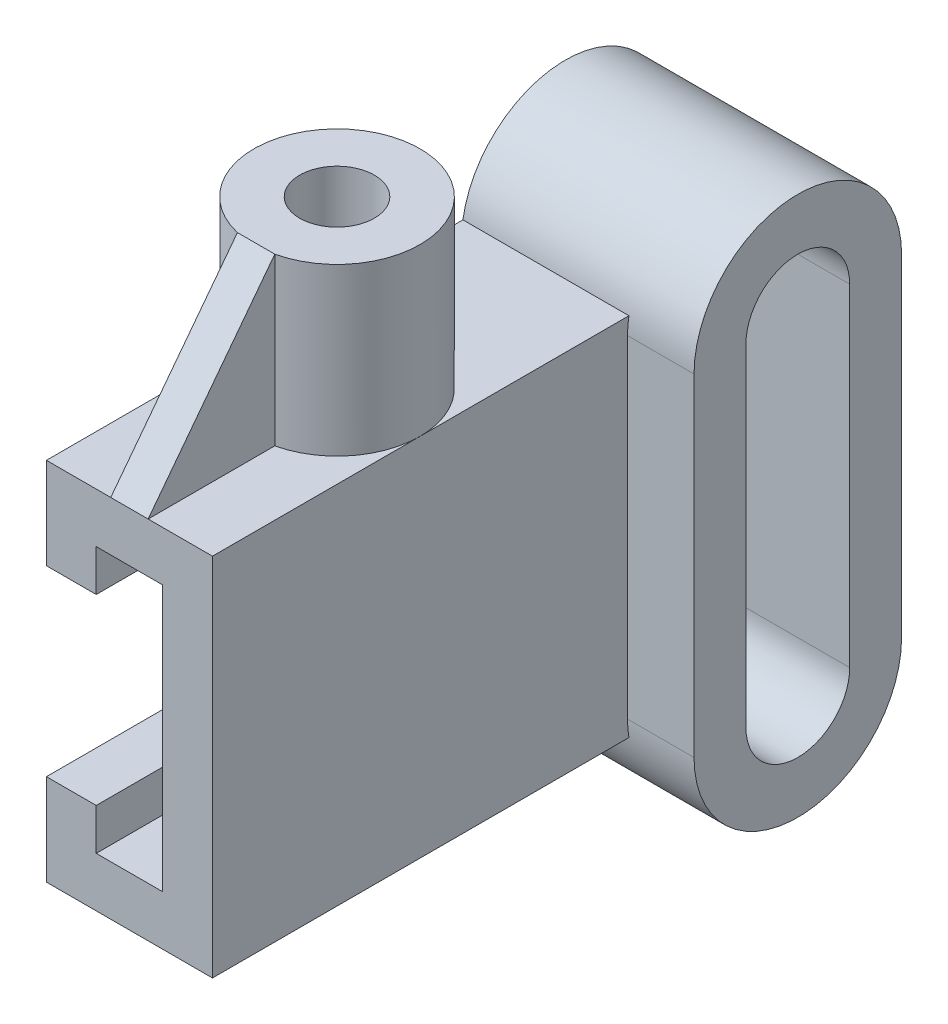
ISO-10303-21;
HEADER;
FILE_DESCRIPTION(('STEP AP214'),'2;1');
FILE_NAME('part.step','',(''),(''),'','','');
FILE_SCHEMA(('AUTOMOTIVE_DESIGN { 1 0 10303 214 1 1 1 1 }'));
ENDSEC;
DATA;
#1=APPLICATION_CONTEXT('core data for automotive mechanical design processes');
#2=APPLICATION_PROTOCOL_DEFINITION('international standard','automotive_design',2000,#1);
#3=PRODUCT_CONTEXT('',#1,'mechanical');
#4=PRODUCT('Part','Part','',(#3));
#5=PRODUCT_RELATED_PRODUCT_CATEGORY('part','',(#4));
#6=PRODUCT_DEFINITION_FORMATION('','',#4);
#7=PRODUCT_DEFINITION_CONTEXT('part definition',#1,'design');
#8=PRODUCT_DEFINITION('design','',#6,#7);
#9=PRODUCT_DEFINITION_SHAPE('','',#8);
#10=(LENGTH_UNIT() NAMED_UNIT(*) SI_UNIT(.MILLI.,.METRE.));
#11=(NAMED_UNIT(*) PLANE_ANGLE_UNIT() SI_UNIT($,.RADIAN.));
#12=(NAMED_UNIT(*) SI_UNIT($,.STERADIAN.) SOLID_ANGLE_UNIT());
#13=UNCERTAINTY_MEASURE_WITH_UNIT(LENGTH_MEASURE(1.E-05),#10,'distance_accuracy_value','');
#14=(GEOMETRIC_REPRESENTATION_CONTEXT(3) GLOBAL_UNCERTAINTY_ASSIGNED_CONTEXT((#13)) GLOBAL_UNIT_ASSIGNED_CONTEXT((#10,
#11,#12)) REPRESENTATION_CONTEXT('',''));
#15=CARTESIAN_POINT('',(0.,0.,0.));
#16=DIRECTION('',(0.,0.,1.));
#17=DIRECTION('',(1.,0.,0.));
#18=AXIS2_PLACEMENT_3D('',#15,#16,#17);
#19=CARTESIAN_POINT('',(-20.,-40.,-74.9999999999999));
#20=DIRECTION('',(1.,0.,0.));
#21=DIRECTION('',(0.,0.,-1.));
#22=AXIS2_PLACEMENT_3D('',#19,#20,#21);
#23=CYLINDRICAL_SURFACE('',#22,25.);
#24=CARTESIAN_POINT('',(20.,-40.,-74.9999999999999));
#25=DIRECTION('',(-1.,0.,0.));
#26=DIRECTION('',(0.,0.,1.));
#27=AXIS2_PLACEMENT_3D('',#24,#25,#26);
#28=CIRCLE('',#27,25.);
#29=CARTESIAN_POINT('',(20.,-44.,-50.3220746414938));
#30=VERTEX_POINT('',#29);
#31=CARTESIAN_POINT('',(20.,-40.,-50.));
#32=VERTEX_POINT('',#31);
#33=EDGE_CURVE('E11',#30,#32,#28,.T.);
#34=ORIENTED_EDGE('',*,*,#33,.F.);
#35=DIRECTION('',(1.,0.,0.));
#36=VECTOR('',#35,1.);
#37=CARTESIAN_POINT('',(-20.,-44.,-50.3220746414938));
#38=LINE('',#37,#36);
#39=CARTESIAN_POINT('',(-20.,-44.,-50.3220746414938));
#40=VERTEX_POINT('',#39);
#41=EDGE_CURVE('E47',#40,#30,#38,.T.);
#42=ORIENTED_EDGE('',*,*,#41,.F.);
#43=CARTESIAN_POINT('',(-20.,-40.,-74.9999999999999));
#44=DIRECTION('',(1.,0.,0.));
#45=DIRECTION('',(0.,0.,-1.));
#46=AXIS2_PLACEMENT_3D('',#43,#44,#45);
#47=CIRCLE('',#46,25.);
#48=CARTESIAN_POINT('',(-20.,-40.,-99.9999999999999));
#49=VERTEX_POINT('',#48);
#50=EDGE_CURVE('E340',#49,#40,#47,.F.);
#51=ORIENTED_EDGE('',*,*,#50,.F.);
#52=DIRECTION('',(1.,0.,0.));
#53=VECTOR('',#52,1.);
#54=CARTESIAN_POINT('',(-20.,-40.,-99.9999999999999));
#55=LINE('',#54,#53);
#56=CARTESIAN_POINT('',(36.,-40.,-99.9999999999999));
#57=VERTEX_POINT('',#56);
#58=EDGE_CURVE('E310',#49,#57,#55,.T.);
#59=ORIENTED_EDGE('',*,*,#58,.T.);
#60=CARTESIAN_POINT('',(36.,-40.,-74.9999999999999));
#61=DIRECTION('',(1.,0.,0.));
#62=DIRECTION('',(0.,0.,-1.));
#63=AXIS2_PLACEMENT_3D('',#60,#61,#62);
#64=CIRCLE('',#63,25.);
#65=CARTESIAN_POINT('',(36.,-40.,-50.));
#66=VERTEX_POINT('',#65);
#67=EDGE_CURVE('E349',#66,#57,#64,.T.);
#68=ORIENTED_EDGE('',*,*,#67,.F.);
#69=DIRECTION('',(-1.,0.,0.));
#70=VECTOR('',#69,1.);
#71=CARTESIAN_POINT('',(36.,-40.,-50.));
#72=LINE('',#71,#70);
#73=EDGE_CURVE('E219',#66,#32,#72,.T.);
#74=ORIENTED_EDGE('',*,*,#73,.T.);
#75=EDGE_LOOP('',(#34,#42,#51,#59,#68,#74));
#76=FACE_BOUND('',#75,.T.);
#77=ADVANCED_FACE('F41',(#76),#23,.T.);
#78=CARTESIAN_POINT('',(-20.,40.,-75.));
#79=DIRECTION('',(1.,0.,0.));
#80=DIRECTION('',(0.,0.,-1.));
#81=AXIS2_PLACEMENT_3D('',#78,#79,#80);
#82=CYLINDRICAL_SURFACE('',#81,25.);
#83=DIRECTION('',(1.,0.,0.));
#84=VECTOR('',#83,1.);
#85=CARTESIAN_POINT('',(-20.,44.,-50.3220746414938));
#86=LINE('',#85,#84);
#87=CARTESIAN_POINT('',(-20.,44.,-50.3220746414938));
#88=VERTEX_POINT('',#87);
#89=CARTESIAN_POINT('',(20.,44.,-50.3220746414938));
#90=VERTEX_POINT('',#89);
#91=EDGE_CURVE('E225',#88,#90,#86,.T.);
#92=ORIENTED_EDGE('',*,*,#91,.T.);
#93=CARTESIAN_POINT('',(20.,40.,-75.));
#94=DIRECTION('',(-1.,0.,0.));
#95=DIRECTION('',(0.,0.,1.));
#96=AXIS2_PLACEMENT_3D('',#93,#94,#95);
#97=CIRCLE('',#96,25.);
#98=CARTESIAN_POINT('',(20.,40.,-50.));
#99=VERTEX_POINT('',#98);
#100=EDGE_CURVE('E224',#90,#99,#97,.F.);
#101=ORIENTED_EDGE('',*,*,#100,.T.);
#102=DIRECTION('',(-1.,0.,0.));
#103=VECTOR('',#102,1.);
#104=CARTESIAN_POINT('',(36.,40.,-50.));
#105=LINE('',#104,#103);
#106=CARTESIAN_POINT('',(36.,40.,-50.));
#107=VERTEX_POINT('',#106);
#108=EDGE_CURVE('E339',#107,#99,#105,.T.);
#109=ORIENTED_EDGE('',*,*,#108,.F.);
#110=CARTESIAN_POINT('',(36.,40.,-75.));
#111=DIRECTION('',(1.,0.,0.));
#112=DIRECTION('',(0.,0.,-1.));
#113=AXIS2_PLACEMENT_3D('',#110,#111,#112);
#114=CIRCLE('',#113,25.);
#115=CARTESIAN_POINT('',(36.,40.,-100.));
#116=VERTEX_POINT('',#115);
#117=EDGE_CURVE('E353',#116,#107,#114,.T.);
#118=ORIENTED_EDGE('',*,*,#117,.F.);
#119=DIRECTION('',(1.,0.,0.));
#120=VECTOR('',#119,1.);
#121=CARTESIAN_POINT('',(-20.,40.,-100.));
#122=LINE('',#121,#120);
#123=CARTESIAN_POINT('',(-20.,40.,-100.));
#124=VERTEX_POINT('',#123);
#125=EDGE_CURVE('E307',#124,#116,#122,.T.);
#126=ORIENTED_EDGE('',*,*,#125,.F.);
#127=CARTESIAN_POINT('',(-20.,40.,-75.));
#128=DIRECTION('',(1.,0.,0.));
#129=DIRECTION('',(0.,0.,-1.));
#130=AXIS2_PLACEMENT_3D('',#127,#128,#129);
#131=CIRCLE('',#130,25.);
#132=EDGE_CURVE('E334',#124,#88,#131,.T.);
#133=ORIENTED_EDGE('',*,*,#132,.T.);
#134=EDGE_LOOP('',(#92,#101,#109,#118,#126,#133));
#135=FACE_BOUND('',#134,.T.);
#136=ADVANCED_FACE('F481',(#135),#82,.T.);
#137=CARTESIAN_POINT('',(-20.,44.,50.));
#138=DIRECTION('',(0.,-1.,0.));
#139=DIRECTION('',(0.,0.,-1.));
#140=AXIS2_PLACEMENT_3D('',#137,#138,#139);
#141=PLANE('',#140);
#142=DIRECTION('',(0.,0.,1.));
#143=VECTOR('',#142,1.);
#144=CARTESIAN_POINT('',(-4.49999999999999,44.,19.4871752699051));
#145=LINE('',#144,#143);
#146=CARTESIAN_POINT('',(-4.49999999999999,44.,19.4871752699051));
#147=VERTEX_POINT('',#146);
#148=CARTESIAN_POINT('',(-4.49999999999999,44.,50.));
#149=VERTEX_POINT('',#148);
#150=EDGE_CURVE('E386',#147,#149,#145,.T.);
#151=ORIENTED_EDGE('',*,*,#150,.F.);
#152=CARTESIAN_POINT('',(0.,44.,0.));
#153=DIRECTION('',(0.,1.,0.));
#154=DIRECTION('',(0.,0.,1.));
#155=AXIS2_PLACEMENT_3D('',#152,#153,#154);
#156=CIRCLE('',#155,20.);
#157=CARTESIAN_POINT('',(-20.,44.,0.));
#158=VERTEX_POINT('',#157);
#159=EDGE_CURVE('E375',#158,#147,#156,.T.);
#160=ORIENTED_EDGE('',*,*,#159,.F.);
#161=DIRECTION('',(0.,0.,-1.));
#162=VECTOR('',#161,1.);
#163=CARTESIAN_POINT('',(-20.,44.,50.));
#164=LINE('',#163,#162);
#165=CARTESIAN_POINT('',(-20.,44.,50.));
#166=VERTEX_POINT('',#165);
#167=EDGE_CURVE('E234',#166,#158,#164,.T.);
#168=ORIENTED_EDGE('',*,*,#167,.F.);
#169=DIRECTION('',(-1.,0.,0.));
#170=VECTOR('',#169,1.);
#171=CARTESIAN_POINT('',(-20.,44.,50.));
#172=LINE('',#171,#170);
#173=EDGE_CURVE('E246',#149,#166,#172,.T.);
#174=ORIENTED_EDGE('',*,*,#173,.F.);
#175=EDGE_LOOP('',(#151,#160,#168,#174));
#176=FACE_BOUND('',#175,.T.);
#177=ADVANCED_FACE('F413',(#176),#141,.F.);
#178=DIRECTION('',(0.,0.,-1.));
#179=VECTOR('',#178,1.);
#180=CARTESIAN_POINT('',(4.50000000000001,44.,19.4871752699051));
#181=LINE('',#180,#179);
#182=CARTESIAN_POINT('',(4.50000000000001,44.,50.));
#183=VERTEX_POINT('',#182);
#184=CARTESIAN_POINT('',(4.50000000000001,44.,19.4871752699051));
#185=VERTEX_POINT('',#184);
#186=EDGE_CURVE('E390',#183,#185,#181,.T.);
#187=ORIENTED_EDGE('',*,*,#186,.F.);
#188=CARTESIAN_POINT('',(20.,44.,50.));
#189=VERTEX_POINT('',#188);
#190=EDGE_CURVE('E243',#189,#183,#172,.T.);
#191=ORIENTED_EDGE('',*,*,#190,.F.);
#192=DIRECTION('',(0.,0.,-1.));
#193=VECTOR('',#192,1.);
#194=CARTESIAN_POINT('',(20.,44.,50.));
#195=LINE('',#194,#193);
#196=CARTESIAN_POINT('',(20.,44.,0.));
#197=VERTEX_POINT('',#196);
#198=EDGE_CURVE('E233',#189,#197,#195,.T.);
#199=ORIENTED_EDGE('',*,*,#198,.T.);
#200=EDGE_CURVE('E373',#185,#197,#156,.T.);
#201=ORIENTED_EDGE('',*,*,#200,.F.);
#202=EDGE_LOOP('',(#187,#191,#199,#201));
#203=FACE_BOUND('',#202,.T.);
#204=ADVANCED_FACE('F452',(#203),#141,.F.);
#205=CARTESIAN_POINT('',(0.,84.,0.));
#206=DIRECTION('',(0.,-1.,0.));
#207=DIRECTION('',(0.,0.,-1.));
#208=AXIS2_PLACEMENT_3D('',#205,#206,#207);
#209=CYLINDRICAL_SURFACE('',#208,20.);
#210=DIRECTION('',(0.,-1.,0.));
#211=VECTOR('',#210,1.);
#212=CARTESIAN_POINT('',(-4.49999999999999,84.,19.4871752699051));
#213=LINE('',#212,#211);
#214=CARTESIAN_POINT('',(-4.49999999999999,84.,19.4871752699051));
#215=VERTEX_POINT('',#214);
#216=EDGE_CURVE('E379',#215,#147,#213,.T.);
#217=ORIENTED_EDGE('',*,*,#216,.F.);
#218=CARTESIAN_POINT('',(0.,84.,0.));
#219=DIRECTION('',(0.,1.,0.));
#220=DIRECTION('',(0.,0.,1.));
#221=AXIS2_PLACEMENT_3D('',#218,#219,#220);
#222=CIRCLE('',#221,20.);
#223=CARTESIAN_POINT('',(4.50000000000001,84.,19.4871752699051));
#224=VERTEX_POINT('',#223);
#225=EDGE_CURVE('E350',#224,#215,#222,.T.);
#226=ORIENTED_EDGE('',*,*,#225,.F.);
#227=DIRECTION('',(0.,-1.,0.));
#228=VECTOR('',#227,1.);
#229=CARTESIAN_POINT('',(4.50000000000001,84.,19.4871752699051));
#230=LINE('',#229,#228);
#231=EDGE_CURVE('E381',#224,#185,#230,.T.);
#232=ORIENTED_EDGE('',*,*,#231,.T.);
#233=ORIENTED_EDGE('',*,*,#200,.T.);
#234=EDGE_CURVE('E367',#197,#158,#156,.T.);
#235=ORIENTED_EDGE('',*,*,#234,.T.);
#236=ORIENTED_EDGE('',*,*,#159,.T.);
#237=EDGE_LOOP('',(#217,#226,#232,#233,#235,#236));
#238=FACE_BOUND('',#237,.T.);
#239=ADVANCED_FACE('F460',(#238),#209,.T.);
#240=CARTESIAN_POINT('',(20.,-44.,50.));
#241=DIRECTION('',(-1.,0.,0.));
#242=DIRECTION('',(0.,0.,1.));
#243=AXIS2_PLACEMENT_3D('',#240,#241,#242);
#244=PLANE('',#243);
#245=DIRECTION('',(0.,-1.,0.));
#246=VECTOR('',#245,1.);
#247=CARTESIAN_POINT('',(20.,0.,-50.));
#248=LINE('',#247,#246);
#249=EDGE_CURVE('E341',#99,#32,#248,.T.);
#250=ORIENTED_EDGE('',*,*,#249,.F.);
#251=ORIENTED_EDGE('',*,*,#100,.F.);
#252=EDGE_CURVE('E61',#197,#90,#195,.T.);
#253=ORIENTED_EDGE('',*,*,#252,.F.);
#254=ORIENTED_EDGE('',*,*,#198,.F.);
#255=DIRECTION('',(0.,1.,0.));
#256=VECTOR('',#255,1.);
#257=CARTESIAN_POINT('',(20.,-44.,50.));
#258=LINE('',#257,#256);
#259=CARTESIAN_POINT('',(20.,-44.,50.));
#260=VERTEX_POINT('',#259);
#261=EDGE_CURVE('E212',#260,#189,#258,.T.);
#262=ORIENTED_EDGE('',*,*,#261,.F.);
#263=DIRECTION('',(0.,0.,-1.));
#264=VECTOR('',#263,1.);
#265=CARTESIAN_POINT('',(20.,-44.,50.));
#266=LINE('',#265,#264);
#267=EDGE_CURVE('E207',#260,#30,#266,.T.);
#268=ORIENTED_EDGE('',*,*,#267,.T.);
#269=ORIENTED_EDGE('',*,*,#33,.T.);
#270=EDGE_LOOP('',(#250,#251,#253,#254,#262,#268,#269));
#271=FACE_BOUND('',#270,.T.);
#272=ADVANCED_FACE('F43',(#271),#244,.F.);
#273=ORIENTED_EDGE('',*,*,#234,.F.);
#274=ORIENTED_EDGE('',*,*,#252,.T.);
#275=ORIENTED_EDGE('',*,*,#91,.F.);
#276=EDGE_CURVE('E236',#158,#88,#164,.T.);
#277=ORIENTED_EDGE('',*,*,#276,.F.);
#278=EDGE_LOOP('',(#273,#274,#275,#277));
#279=FACE_BOUND('',#278,.T.);
#280=ADVANCED_FACE('F471',(#279),#141,.F.);
#281=CARTESIAN_POINT('',(-20.,-44.,50.));
#282=DIRECTION('',(1.,0.,0.));
#283=DIRECTION('',(0.,0.,-1.));
#284=AXIS2_PLACEMENT_3D('',#281,#282,#283);
#285=PLANE('',#284);
#286=ORIENTED_EDGE('',*,*,#50,.T.);
#287=DIRECTION('',(0.,0.,-1.));
#288=VECTOR('',#287,1.);
#289=CARTESIAN_POINT('',(-20.,-44.,50.));
#290=LINE('',#289,#288);
#291=CARTESIAN_POINT('',(-20.,-44.,50.));
#292=VERTEX_POINT('',#291);
#293=EDGE_CURVE('E57',#292,#40,#290,.T.);
#294=ORIENTED_EDGE('',*,*,#293,.F.);
#295=DIRECTION('',(0.,-1.,0.));
#296=VECTOR('',#295,1.);
#297=CARTESIAN_POINT('',(-20.,-44.,50.));
#298=LINE('',#297,#296);
#299=CARTESIAN_POINT('',(-20.,-22.,50.));
#300=VERTEX_POINT('',#299);
#301=EDGE_CURVE('E245',#300,#292,#298,.T.);
#302=ORIENTED_EDGE('',*,*,#301,.F.);
#303=DIRECTION('',(0.,0.,1.));
#304=VECTOR('',#303,1.);
#305=CARTESIAN_POINT('',(-20.,-22.,-50.));
#306=LINE('',#305,#304);
#307=CARTESIAN_POINT('',(-20.,-22.,-50.));
#308=VERTEX_POINT('',#307);
#309=EDGE_CURVE('E248',#308,#300,#306,.T.);
#310=ORIENTED_EDGE('',*,*,#309,.F.);
#311=DIRECTION('',(0.,1.,0.));
#312=VECTOR('',#311,1.);
#313=CARTESIAN_POINT('',(-20.,0.,-50.));
#314=LINE('',#313,#312);
#315=CARTESIAN_POINT('',(-20.,22.,-50.));
#316=VERTEX_POINT('',#315);
#317=EDGE_CURVE('E327',#308,#316,#314,.T.);
#318=ORIENTED_EDGE('',*,*,#317,.T.);
#319=DIRECTION('',(0.,0.,1.));
#320=VECTOR('',#319,1.);
#321=CARTESIAN_POINT('',(-20.,22.,-50.));
#322=LINE('',#321,#320);
#323=CARTESIAN_POINT('',(-20.,22.,50.));
#324=VERTEX_POINT('',#323);
#325=EDGE_CURVE('E247',#316,#324,#322,.T.);
#326=ORIENTED_EDGE('',*,*,#325,.T.);
#327=EDGE_CURVE('E237',#166,#324,#298,.T.);
#328=ORIENTED_EDGE('',*,*,#327,.F.);
#329=ORIENTED_EDGE('',*,*,#167,.T.);
#330=ORIENTED_EDGE('',*,*,#276,.T.);
#331=ORIENTED_EDGE('',*,*,#132,.F.);
#332=DIRECTION('',(0.,-1.,0.));
#333=VECTOR('',#332,1.);
#334=CARTESIAN_POINT('',(-20.,0.,-99.9999999999999));
#335=LINE('',#334,#333);
#336=EDGE_CURVE('E333',#124,#49,#335,.T.);
#337=ORIENTED_EDGE('',*,*,#336,.T.);
#338=EDGE_LOOP('',(#286,#294,#302,#310,#318,#326,#328,#329,#330,#331,#337));
#339=FACE_BOUND('',#338,.T.);
#340=DIRECTION('',(0.,-1.,0.));
#341=VECTOR('',#340,1.);
#342=CARTESIAN_POINT('',(-20.,0.,-87.4999999999999));
#343=LINE('',#342,#341);
#344=CARTESIAN_POINT('',(-20.,40.,-87.5));
#345=VERTEX_POINT('',#344);
#346=CARTESIAN_POINT('',(-20.,-40.,-87.4999999999999));
#347=VERTEX_POINT('',#346);
#348=EDGE_CURVE('E326',#345,#347,#343,.T.);
#349=ORIENTED_EDGE('',*,*,#348,.F.);
#350=CARTESIAN_POINT('',(-20.,40.,-75.));
#351=DIRECTION('',(1.,0.,0.));
#352=DIRECTION('',(0.,0.,-1.));
#353=AXIS2_PLACEMENT_3D('',#350,#351,#352);
#354=CIRCLE('',#353,12.5);
#355=CARTESIAN_POINT('',(-20.,40.,-62.5));
#356=VERTEX_POINT('',#355);
#357=EDGE_CURVE('E309',#345,#356,#354,.T.);
#358=ORIENTED_EDGE('',*,*,#357,.T.);
#359=DIRECTION('',(0.,-1.,0.));
#360=VECTOR('',#359,1.);
#361=CARTESIAN_POINT('',(-20.,0.,-62.4999999999999));
#362=LINE('',#361,#360);
#363=CARTESIAN_POINT('',(-20.,-40.,-62.4999999999999));
#364=VERTEX_POINT('',#363);
#365=EDGE_CURVE('E322',#356,#364,#362,.T.);
#366=ORIENTED_EDGE('',*,*,#365,.T.);
#367=CARTESIAN_POINT('',(-20.,-40.,-74.9999999999999));
#368=DIRECTION('',(1.,0.,0.));
#369=DIRECTION('',(0.,0.,-1.));
#370=AXIS2_PLACEMENT_3D('',#367,#368,#369);
#371=CIRCLE('',#370,12.5);
#372=EDGE_CURVE('E324',#347,#364,#371,.F.);
#373=ORIENTED_EDGE('',*,*,#372,.F.);
#374=EDGE_LOOP('',(#349,#358,#366,#373));
#375=FACE_BOUND('',#374,.T.);
#376=ADVANCED_FACE('F419',(#339,#375),#285,.F.);
#377=CARTESIAN_POINT('',(-20.,-44.,50.));
#378=DIRECTION('',(0.,1.,0.));
#379=DIRECTION('',(0.,0.,1.));
#380=AXIS2_PLACEMENT_3D('',#377,#378,#379);
#381=PLANE('',#380);
#382=ORIENTED_EDGE('',*,*,#293,.T.);
#383=ORIENTED_EDGE('',*,*,#41,.T.);
#384=ORIENTED_EDGE('',*,*,#267,.F.);
#385=DIRECTION('',(1.,0.,0.));
#386=VECTOR('',#385,1.);
#387=CARTESIAN_POINT('',(-20.,-44.,50.));
#388=LINE('',#387,#386);
#389=EDGE_CURVE('E215',#292,#260,#388,.T.);
#390=ORIENTED_EDGE('',*,*,#389,.F.);
#391=EDGE_LOOP('',(#382,#383,#384,#390));
#392=FACE_BOUND('',#391,.T.);
#393=ADVANCED_FACE('F222',(#392),#381,.F.);
#394=CARTESIAN_POINT('',(0.,0.,50.));
#395=DIRECTION('',(0.,0.,-1.));
#396=DIRECTION('',(-1.,0.,0.));
#397=AXIS2_PLACEMENT_3D('',#394,#395,#396);
#398=PLANE('',#397);
#399=ORIENTED_EDGE('',*,*,#190,.T.);
#400=DIRECTION('',(-1.,0.,0.));
#401=VECTOR('',#400,1.);
#402=CARTESIAN_POINT('',(35.5,44.,50.));
#403=LINE('',#402,#401);
#404=EDGE_CURVE('E395',#183,#149,#403,.T.);
#405=ORIENTED_EDGE('',*,*,#404,.T.);
#406=ORIENTED_EDGE('',*,*,#173,.T.);
#407=ORIENTED_EDGE('',*,*,#327,.T.);
#408=DIRECTION('',(-1.,0.,0.));
#409=VECTOR('',#408,1.);
#410=CARTESIAN_POINT('',(-20.,22.,50.));
#411=LINE('',#410,#409);
#412=CARTESIAN_POINT('',(-8.,22.,50.));
#413=VERTEX_POINT('',#412);
#414=EDGE_CURVE('E267',#413,#324,#411,.T.);
#415=ORIENTED_EDGE('',*,*,#414,.F.);
#416=DIRECTION('',(0.,-1.,0.));
#417=VECTOR('',#416,1.);
#418=CARTESIAN_POINT('',(-8.,22.,50.));
#419=LINE('',#418,#417);
#420=CARTESIAN_POINT('',(-8.,32.,50.));
#421=VERTEX_POINT('',#420);
#422=EDGE_CURVE('E266',#421,#413,#419,.T.);
#423=ORIENTED_EDGE('',*,*,#422,.F.);
#424=DIRECTION('',(-1.,0.,0.));
#425=VECTOR('',#424,1.);
#426=CARTESIAN_POINT('',(-8.,32.,50.));
#427=LINE('',#426,#425);
#428=CARTESIAN_POINT('',(7.99999999999999,32.,50.));
#429=VERTEX_POINT('',#428);
#430=EDGE_CURVE('E275',#429,#421,#427,.T.);
#431=ORIENTED_EDGE('',*,*,#430,.F.);
#432=DIRECTION('',(0.,1.,0.));
#433=VECTOR('',#432,1.);
#434=CARTESIAN_POINT('',(7.99999999999999,32.,50.));
#435=LINE('',#434,#433);
#436=CARTESIAN_POINT('',(7.99999999999999,-32.,50.));
#437=VERTEX_POINT('',#436);
#438=EDGE_CURVE('E273',#437,#429,#435,.T.);
#439=ORIENTED_EDGE('',*,*,#438,.F.);
#440=DIRECTION('',(1.,0.,0.));
#441=VECTOR('',#440,1.);
#442=CARTESIAN_POINT('',(7.99999999999999,-32.,50.));
#443=LINE('',#442,#441);
#444=CARTESIAN_POINT('',(-8.,-32.,50.));
#445=VERTEX_POINT('',#444);
#446=EDGE_CURVE('E279',#445,#437,#443,.T.);
#447=ORIENTED_EDGE('',*,*,#446,.F.);
#448=DIRECTION('',(0.,-1.,0.));
#449=VECTOR('',#448,1.);
#450=CARTESIAN_POINT('',(-8.,-32.,50.));
#451=LINE('',#450,#449);
#452=CARTESIAN_POINT('',(-8.,-22.,50.));
#453=VERTEX_POINT('',#452);
#454=EDGE_CURVE('E281',#453,#445,#451,.T.);
#455=ORIENTED_EDGE('',*,*,#454,.F.);
#456=DIRECTION('',(1.,0.,0.));
#457=VECTOR('',#456,1.);
#458=CARTESIAN_POINT('',(-8.,-22.,50.));
#459=LINE('',#458,#457);
#460=EDGE_CURVE('E282',#300,#453,#459,.T.);
#461=ORIENTED_EDGE('',*,*,#460,.F.);
#462=ORIENTED_EDGE('',*,*,#301,.T.);
#463=ORIENTED_EDGE('',*,*,#389,.T.);
#464=ORIENTED_EDGE('',*,*,#261,.T.);
#465=EDGE_LOOP('',(#399,#405,#406,#407,#415,#423,#431,#439,#447,#455,#461,#462,#463,#464));
#466=FACE_BOUND('',#465,.T.);
#467=ADVANCED_FACE('F403',(#466),#398,.F.);
#468=CARTESIAN_POINT('',(-20.,22.,-50.));
#469=DIRECTION('',(0.,1.,0.));
#470=DIRECTION('',(-1.,0.,0.));
#471=AXIS2_PLACEMENT_3D('',#468,#469,#470);
#472=PLANE('',#471);
#473=ORIENTED_EDGE('',*,*,#414,.T.);
#474=ORIENTED_EDGE('',*,*,#325,.F.);
#475=DIRECTION('',(-1.,0.,0.));
#476=VECTOR('',#475,1.);
#477=CARTESIAN_POINT('',(-20.,22.,-50.));
#478=LINE('',#477,#476);
#479=CARTESIAN_POINT('',(-8.,22.,-50.));
#480=VERTEX_POINT('',#479);
#481=EDGE_CURVE('E255',#480,#316,#478,.T.);
#482=ORIENTED_EDGE('',*,*,#481,.F.);
#483=DIRECTION('',(0.,0.,1.));
#484=VECTOR('',#483,1.);
#485=CARTESIAN_POINT('',(-8.,22.,-50.));
#486=LINE('',#485,#484);
#487=EDGE_CURVE('E265',#480,#413,#486,.T.);
#488=ORIENTED_EDGE('',*,*,#487,.T.);
#489=EDGE_LOOP('',(#473,#474,#482,#488));
#490=FACE_BOUND('',#489,.T.);
#491=ADVANCED_FACE('F421',(#490),#472,.F.);
#492=CARTESIAN_POINT('',(-8.,22.,-50.));
#493=DIRECTION('',(-1.,0.,0.));
#494=DIRECTION('',(0.,0.,1.));
#495=AXIS2_PLACEMENT_3D('',#492,#493,#494);
#496=PLANE('',#495);
#497=ORIENTED_EDGE('',*,*,#422,.T.);
#498=ORIENTED_EDGE('',*,*,#487,.F.);
#499=DIRECTION('',(0.,-1.,0.));
#500=VECTOR('',#499,1.);
#501=CARTESIAN_POINT('',(-8.,22.,-50.));
#502=LINE('',#501,#500);
#503=CARTESIAN_POINT('',(-8.,32.,-50.));
#504=VERTEX_POINT('',#503);
#505=EDGE_CURVE('E288',#504,#480,#502,.T.);
#506=ORIENTED_EDGE('',*,*,#505,.F.);
#507=DIRECTION('',(0.,0.,1.));
#508=VECTOR('',#507,1.);
#509=CARTESIAN_POINT('',(-8.,32.,-50.));
#510=LINE('',#509,#508);
#511=EDGE_CURVE('E258',#504,#421,#510,.T.);
#512=ORIENTED_EDGE('',*,*,#511,.T.);
#513=EDGE_LOOP('',(#497,#498,#506,#512));
#514=FACE_BOUND('',#513,.T.);
#515=ADVANCED_FACE('F430',(#514),#496,.F.);
#516=CARTESIAN_POINT('',(-8.,32.,-50.));
#517=DIRECTION('',(0.,1.,0.));
#518=DIRECTION('',(0.,0.,1.));
#519=AXIS2_PLACEMENT_3D('',#516,#517,#518);
#520=PLANE('',#519);
#521=ORIENTED_EDGE('',*,*,#430,.T.);
#522=ORIENTED_EDGE('',*,*,#511,.F.);
#523=DIRECTION('',(-1.,0.,0.));
#524=VECTOR('',#523,1.);
#525=CARTESIAN_POINT('',(-8.,32.,-50.));
#526=LINE('',#525,#524);
#527=CARTESIAN_POINT('',(7.99999999999999,32.,-50.));
#528=VERTEX_POINT('',#527);
#529=EDGE_CURVE('E291',#528,#504,#526,.T.);
#530=ORIENTED_EDGE('',*,*,#529,.F.);
#531=DIRECTION('',(0.,0.,1.));
#532=VECTOR('',#531,1.);
#533=CARTESIAN_POINT('',(7.99999999999999,32.,-50.));
#534=LINE('',#533,#532);
#535=EDGE_CURVE('E259',#528,#429,#534,.T.);
#536=ORIENTED_EDGE('',*,*,#535,.T.);
#537=EDGE_LOOP('',(#521,#522,#530,#536));
#538=FACE_BOUND('',#537,.T.);
#539=ADVANCED_FACE('F427',(#538),#520,.F.);
#540=CARTESIAN_POINT('',(7.99999999999999,32.,-50.));
#541=DIRECTION('',(1.,0.,0.));
#542=DIRECTION('',(0.,0.,-1.));
#543=AXIS2_PLACEMENT_3D('',#540,#541,#542);
#544=PLANE('',#543);
#545=ORIENTED_EDGE('',*,*,#438,.T.);
#546=ORIENTED_EDGE('',*,*,#535,.F.);
#547=DIRECTION('',(0.,1.,0.));
#548=VECTOR('',#547,1.);
#549=CARTESIAN_POINT('',(7.99999999999999,32.,-50.));
#550=LINE('',#549,#548);
#551=CARTESIAN_POINT('',(7.99999999999999,-32.,-50.));
#552=VERTEX_POINT('',#551);
#553=EDGE_CURVE('E298',#552,#528,#550,.T.);
#554=ORIENTED_EDGE('',*,*,#553,.F.);
#555=DIRECTION('',(0.,0.,1.));
#556=VECTOR('',#555,1.);
#557=CARTESIAN_POINT('',(7.99999999999999,-32.,-50.));
#558=LINE('',#557,#556);
#559=EDGE_CURVE('E257',#552,#437,#558,.T.);
#560=ORIENTED_EDGE('',*,*,#559,.T.);
#561=EDGE_LOOP('',(#545,#546,#554,#560));
#562=FACE_BOUND('',#561,.T.);
#563=ADVANCED_FACE('F434',(#562),#544,.F.);
#564=CARTESIAN_POINT('',(7.99999999999999,-32.,-50.));
#565=DIRECTION('',(0.,-1.,0.));
#566=DIRECTION('',(0.,0.,-1.));
#567=AXIS2_PLACEMENT_3D('',#564,#565,#566);
#568=PLANE('',#567);
#569=ORIENTED_EDGE('',*,*,#446,.T.);
#570=ORIENTED_EDGE('',*,*,#559,.F.);
#571=DIRECTION('',(1.,0.,0.));
#572=VECTOR('',#571,1.);
#573=CARTESIAN_POINT('',(7.99999999999999,-32.,-50.));
#574=LINE('',#573,#572);
#575=CARTESIAN_POINT('',(-8.,-32.,-50.));
#576=VERTEX_POINT('',#575);
#577=EDGE_CURVE('E299',#576,#552,#574,.T.);
#578=ORIENTED_EDGE('',*,*,#577,.F.);
#579=DIRECTION('',(0.,0.,1.));
#580=VECTOR('',#579,1.);
#581=CARTESIAN_POINT('',(-8.,-32.,-50.));
#582=LINE('',#581,#580);
#583=EDGE_CURVE('E251',#576,#445,#582,.T.);
#584=ORIENTED_EDGE('',*,*,#583,.T.);
#585=EDGE_LOOP('',(#569,#570,#578,#584));
#586=FACE_BOUND('',#585,.T.);
#587=ADVANCED_FACE('F437',(#586),#568,.F.);
#588=CARTESIAN_POINT('',(-8.,-32.,-50.));
#589=DIRECTION('',(-1.,0.,0.));
#590=DIRECTION('',(0.,0.,1.));
#591=AXIS2_PLACEMENT_3D('',#588,#589,#590);
#592=PLANE('',#591);
#593=ORIENTED_EDGE('',*,*,#454,.T.);
#594=ORIENTED_EDGE('',*,*,#583,.F.);
#595=DIRECTION('',(0.,-1.,0.));
#596=VECTOR('',#595,1.);
#597=CARTESIAN_POINT('',(-8.,-32.,-50.));
#598=LINE('',#597,#596);
#599=CARTESIAN_POINT('',(-8.,-22.,-50.));
#600=VERTEX_POINT('',#599);
#601=EDGE_CURVE('E305',#600,#576,#598,.T.);
#602=ORIENTED_EDGE('',*,*,#601,.F.);
#603=DIRECTION('',(0.,0.,1.));
#604=VECTOR('',#603,1.);
#605=CARTESIAN_POINT('',(-8.,-22.,-50.));
#606=LINE('',#605,#604);
#607=EDGE_CURVE('E252',#600,#453,#606,.T.);
#608=ORIENTED_EDGE('',*,*,#607,.T.);
#609=EDGE_LOOP('',(#593,#594,#602,#608));
#610=FACE_BOUND('',#609,.T.);
#611=ADVANCED_FACE('F445',(#610),#592,.F.);
#612=CARTESIAN_POINT('',(-8.,-22.,-50.));
#613=DIRECTION('',(0.,-1.,0.));
#614=DIRECTION('',(0.,0.,-1.));
#615=AXIS2_PLACEMENT_3D('',#612,#613,#614);
#616=PLANE('',#615);
#617=ORIENTED_EDGE('',*,*,#460,.T.);
#618=ORIENTED_EDGE('',*,*,#607,.F.);
#619=DIRECTION('',(1.,0.,0.));
#620=VECTOR('',#619,1.);
#621=CARTESIAN_POINT('',(-8.,-22.,-50.));
#622=LINE('',#621,#620);
#623=EDGE_CURVE('E270',#308,#600,#622,.T.);
#624=ORIENTED_EDGE('',*,*,#623,.F.);
#625=ORIENTED_EDGE('',*,*,#309,.T.);
#626=EDGE_LOOP('',(#617,#618,#624,#625));
#627=FACE_BOUND('',#626,.T.);
#628=ADVANCED_FACE('F510',(#627),#616,.F.);
#629=CARTESIAN_POINT('',(-20.,0.,-50.));
#630=DIRECTION('',(0.,0.,-1.));
#631=DIRECTION('',(-1.,0.,0.));
#632=AXIS2_PLACEMENT_3D('',#629,#630,#631);
#633=PLANE('',#632);
#634=ORIENTED_EDGE('',*,*,#505,.T.);
#635=ORIENTED_EDGE('',*,*,#481,.T.);
#636=ORIENTED_EDGE('',*,*,#317,.F.);
#637=ORIENTED_EDGE('',*,*,#623,.T.);
#638=ORIENTED_EDGE('',*,*,#601,.T.);
#639=ORIENTED_EDGE('',*,*,#577,.T.);
#640=ORIENTED_EDGE('',*,*,#553,.T.);
#641=ORIENTED_EDGE('',*,*,#529,.T.);
#642=EDGE_LOOP('',(#634,#635,#636,#637,#638,#639,#640,#641));
#643=FACE_BOUND('',#642,.T.);
#644=ADVANCED_FACE('F509',(#643),#633,.F.);
#645=CARTESIAN_POINT('',(-20.,0.,-87.4999999999999));
#646=DIRECTION('',(0.,0.,1.));
#647=DIRECTION('',(0.,-1.,0.));
#648=AXIS2_PLACEMENT_3D('',#645,#646,#647);
#649=PLANE('',#648);
#650=DIRECTION('',(1.,0.,0.));
#651=VECTOR('',#650,1.);
#652=CARTESIAN_POINT('',(-20.,-40.,-87.4999999999999));
#653=LINE('',#652,#651);
#654=CARTESIAN_POINT('',(36.,-40.,-87.4999999999999));
#655=VERTEX_POINT('',#654);
#656=EDGE_CURVE('E315',#347,#655,#653,.T.);
#657=ORIENTED_EDGE('',*,*,#656,.T.);
#658=DIRECTION('',(0.,-1.,0.));
#659=VECTOR('',#658,1.);
#660=CARTESIAN_POINT('',(36.,0.,-87.4999999999999));
#661=LINE('',#660,#659);
#662=CARTESIAN_POINT('',(36.,40.,-87.5));
#663=VERTEX_POINT('',#662);
#664=EDGE_CURVE('E364',#663,#655,#661,.T.);
#665=ORIENTED_EDGE('',*,*,#664,.F.);
#666=DIRECTION('',(1.,0.,0.));
#667=VECTOR('',#666,1.);
#668=CARTESIAN_POINT('',(-20.,40.,-87.5));
#669=LINE('',#668,#667);
#670=EDGE_CURVE('E289',#345,#663,#669,.T.);
#671=ORIENTED_EDGE('',*,*,#670,.F.);
#672=ORIENTED_EDGE('',*,*,#348,.T.);
#673=EDGE_LOOP('',(#657,#665,#671,#672));
#674=FACE_BOUND('',#673,.T.);
#675=ADVANCED_FACE('F669',(#674),#649,.T.);
#676=CARTESIAN_POINT('',(-20.,40.,-75.));
#677=DIRECTION('',(1.,0.,0.));
#678=DIRECTION('',(0.,0.,-1.));
#679=AXIS2_PLACEMENT_3D('',#676,#677,#678);
#680=CYLINDRICAL_SURFACE('',#679,12.5);
#681=ORIENTED_EDGE('',*,*,#670,.T.);
#682=CARTESIAN_POINT('',(36.,40.,-75.));
#683=DIRECTION('',(1.,0.,0.));
#684=DIRECTION('',(0.,0.,-1.));
#685=AXIS2_PLACEMENT_3D('',#682,#683,#684);
#686=CIRCLE('',#685,12.5);
#687=CARTESIAN_POINT('',(36.,40.,-62.5));
#688=VERTEX_POINT('',#687);
#689=EDGE_CURVE('E346',#688,#663,#686,.F.);
#690=ORIENTED_EDGE('',*,*,#689,.F.);
#691=DIRECTION('',(1.,0.,0.));
#692=VECTOR('',#691,1.);
#693=CARTESIAN_POINT('',(-20.,40.,-62.5));
#694=LINE('',#693,#692);
#695=EDGE_CURVE('E317',#356,#688,#694,.T.);
#696=ORIENTED_EDGE('',*,*,#695,.F.);
#697=ORIENTED_EDGE('',*,*,#357,.F.);
#698=EDGE_LOOP('',(#681,#690,#696,#697));
#699=FACE_BOUND('',#698,.T.);
#700=ADVANCED_FACE('F682',(#699),#680,.F.);
#701=CARTESIAN_POINT('',(-20.,0.,-62.4999999999999));
#702=DIRECTION('',(0.,0.,1.));
#703=DIRECTION('',(0.,-1.,0.));
#704=AXIS2_PLACEMENT_3D('',#701,#702,#703);
#705=PLANE('',#704);
#706=ORIENTED_EDGE('',*,*,#695,.T.);
#707=DIRECTION('',(0.,1.,0.));
#708=VECTOR('',#707,1.);
#709=CARTESIAN_POINT('',(36.,0.,-62.4999999999999));
#710=LINE('',#709,#708);
#711=CARTESIAN_POINT('',(36.,-40.,-62.4999999999999));
#712=VERTEX_POINT('',#711);
#713=EDGE_CURVE('E356',#712,#688,#710,.T.);
#714=ORIENTED_EDGE('',*,*,#713,.F.);
#715=DIRECTION('',(1.,0.,0.));
#716=VECTOR('',#715,1.);
#717=CARTESIAN_POINT('',(-20.,-40.,-62.4999999999999));
#718=LINE('',#717,#716);
#719=EDGE_CURVE('E313',#364,#712,#718,.T.);
#720=ORIENTED_EDGE('',*,*,#719,.F.);
#721=ORIENTED_EDGE('',*,*,#365,.F.);
#722=EDGE_LOOP('',(#706,#714,#720,#721));
#723=FACE_BOUND('',#722,.T.);
#724=ADVANCED_FACE('F696',(#723),#705,.F.);
#725=CARTESIAN_POINT('',(-20.,0.,-99.9999999999999));
#726=DIRECTION('',(0.,0.,1.));
#727=DIRECTION('',(0.,-1.,0.));
#728=AXIS2_PLACEMENT_3D('',#725,#726,#727);
#729=PLANE('',#728);
#730=ORIENTED_EDGE('',*,*,#125,.T.);
#731=DIRECTION('',(0.,1.,0.));
#732=VECTOR('',#731,1.);
#733=CARTESIAN_POINT('',(36.,0.,-99.9999999999999));
#734=LINE('',#733,#732);
#735=EDGE_CURVE('E344',#57,#116,#734,.T.);
#736=ORIENTED_EDGE('',*,*,#735,.F.);
#737=ORIENTED_EDGE('',*,*,#58,.F.);
#738=ORIENTED_EDGE('',*,*,#336,.F.);
#739=EDGE_LOOP('',(#730,#736,#737,#738));
#740=FACE_BOUND('',#739,.T.);
#741=ADVANCED_FACE('F494',(#740),#729,.F.);
#742=CARTESIAN_POINT('',(-20.,-40.,-74.9999999999999));
#743=DIRECTION('',(1.,0.,0.));
#744=DIRECTION('',(0.,0.,-1.));
#745=AXIS2_PLACEMENT_3D('',#742,#743,#744);
#746=CYLINDRICAL_SURFACE('',#745,12.5);
#747=ORIENTED_EDGE('',*,*,#719,.T.);
#748=CARTESIAN_POINT('',(36.,-40.,-74.9999999999999));
#749=DIRECTION('',(1.,0.,0.));
#750=DIRECTION('',(0.,0.,-1.));
#751=AXIS2_PLACEMENT_3D('',#748,#749,#750);
#752=CIRCLE('',#751,12.5);
#753=EDGE_CURVE('E363',#655,#712,#752,.F.);
#754=ORIENTED_EDGE('',*,*,#753,.F.);
#755=ORIENTED_EDGE('',*,*,#656,.F.);
#756=ORIENTED_EDGE('',*,*,#372,.T.);
#757=EDGE_LOOP('',(#747,#754,#755,#756));
#758=FACE_BOUND('',#757,.T.);
#759=ADVANCED_FACE('F532',(#758),#746,.F.);
#760=CARTESIAN_POINT('',(36.,0.,-50.));
#761=DIRECTION('',(0.,0.,-1.));
#762=DIRECTION('',(0.,1.,0.));
#763=AXIS2_PLACEMENT_3D('',#760,#761,#762);
#764=PLANE('',#763);
#765=ORIENTED_EDGE('',*,*,#249,.T.);
#766=ORIENTED_EDGE('',*,*,#73,.F.);
#767=DIRECTION('',(0.,-1.,0.));
#768=VECTOR('',#767,1.);
#769=CARTESIAN_POINT('',(36.,0.,-50.));
#770=LINE('',#769,#768);
#771=EDGE_CURVE('E355',#107,#66,#770,.T.);
#772=ORIENTED_EDGE('',*,*,#771,.F.);
#773=ORIENTED_EDGE('',*,*,#108,.T.);
#774=EDGE_LOOP('',(#765,#766,#772,#773));
#775=FACE_BOUND('',#774,.T.);
#776=ADVANCED_FACE('F530',(#775),#764,.F.);
#777=CARTESIAN_POINT('',(36.,0.,0.));
#778=DIRECTION('',(1.,0.,0.));
#779=DIRECTION('',(0.,0.,-1.));
#780=AXIS2_PLACEMENT_3D('',#777,#778,#779);
#781=PLANE('',#780);
#782=ORIENTED_EDGE('',*,*,#689,.T.);
#783=ORIENTED_EDGE('',*,*,#664,.T.);
#784=ORIENTED_EDGE('',*,*,#753,.T.);
#785=ORIENTED_EDGE('',*,*,#713,.T.);
#786=EDGE_LOOP('',(#782,#783,#784,#785));
#787=FACE_BOUND('',#786,.T.);
#788=ORIENTED_EDGE('',*,*,#117,.T.);
#789=ORIENTED_EDGE('',*,*,#771,.T.);
#790=ORIENTED_EDGE('',*,*,#67,.T.);
#791=ORIENTED_EDGE('',*,*,#735,.T.);
#792=EDGE_LOOP('',(#788,#789,#790,#791));
#793=FACE_BOUND('',#792,.T.);
#794=ADVANCED_FACE('F465',(#787,#793),#781,.T.);
#795=CARTESIAN_POINT('',(0.,84.,0.));
#796=DIRECTION('',(0.,1.,0.));
#797=DIRECTION('',(0.,0.,1.));
#798=AXIS2_PLACEMENT_3D('',#795,#796,#797);
#799=PLANE('',#798);
#800=DIRECTION('',(-1.,0.,0.));
#801=VECTOR('',#800,1.);
#802=CARTESIAN_POINT('',(35.5,84.,19.4871752699051));
#803=LINE('',#802,#801);
#804=EDGE_CURVE('E393',#224,#215,#803,.T.);
#805=ORIENTED_EDGE('',*,*,#804,.F.);
#806=ORIENTED_EDGE('',*,*,#225,.T.);
#807=EDGE_LOOP('',(#805,#806));
#808=FACE_BOUND('',#807,.T.);
#809=CARTESIAN_POINT('',(0.,84.,0.));
#810=DIRECTION('',(0.,1.,0.));
#811=DIRECTION('',(0.,0.,1.));
#812=AXIS2_PLACEMENT_3D('',#809,#810,#811);
#813=CIRCLE('',#812,9.);
#814=CARTESIAN_POINT('',(0.,84.,9.));
#815=VERTEX_POINT('',#814);
#816=EDGE_CURVE('E378',#815,#815,#813,.T.);
#817=ORIENTED_EDGE('',*,*,#816,.F.);
#818=EDGE_LOOP('',(#817));
#819=FACE_BOUND('',#818,.T.);
#820=ADVANCED_FACE('F457',(#808,#819),#799,.T.);
#821=CARTESIAN_POINT('',(0.,84.,0.));
#822=DIRECTION('',(0.,-1.,0.));
#823=DIRECTION('',(0.,0.,-1.));
#824=AXIS2_PLACEMENT_3D('',#821,#822,#823);
#825=CYLINDRICAL_SURFACE('',#824,9.);
#826=ORIENTED_EDGE('',*,*,#816,.T.);
#827=EDGE_LOOP('',(#826));
#828=FACE_BOUND('',#827,.T.);
#829=CARTESIAN_POINT('',(0.,44.,0.));
#830=DIRECTION('',(0.,1.,0.));
#831=DIRECTION('',(0.,0.,1.));
#832=AXIS2_PLACEMENT_3D('',#829,#830,#831);
#833=CIRCLE('',#832,9.);
#834=CARTESIAN_POINT('',(0.,44.,9.));
#835=VERTEX_POINT('',#834);
#836=EDGE_CURVE('E376',#835,#835,#833,.T.);
#837=ORIENTED_EDGE('',*,*,#836,.F.);
#838=EDGE_LOOP('',(#837));
#839=FACE_BOUND('',#838,.T.);
#840=ADVANCED_FACE('F464',(#828,#839),#825,.F.);
#841=ORIENTED_EDGE('',*,*,#836,.T.);
#842=EDGE_LOOP('',(#841));
#843=FACE_BOUND('',#842,.T.);
#844=ADVANCED_FACE('F469',(#843),#141,.F.);
#845=CARTESIAN_POINT('',(-4.49999999999999,84.,19.4871752699051));
#846=DIRECTION('',(1.,0.,0.));
#847=DIRECTION('',(0.,0.,-1.));
#848=AXIS2_PLACEMENT_3D('',#845,#846,#847);
#849=PLANE('',#848);
#850=ORIENTED_EDGE('',*,*,#150,.T.);
#851=DIRECTION('',(0.,-0.795080555989343,0.606503841280232));
#852=VECTOR('',#851,1.);
#853=CARTESIAN_POINT('',(-4.49999999999999,84.,19.4871752699051));
#854=LINE('',#853,#852);
#855=EDGE_CURVE('E394',#215,#149,#854,.T.);
#856=ORIENTED_EDGE('',*,*,#855,.F.);
#857=ORIENTED_EDGE('',*,*,#216,.T.);
#858=EDGE_LOOP('',(#850,#856,#857));
#859=FACE_BOUND('',#858,.T.);
#860=ADVANCED_FACE('F406',(#859),#849,.F.);
#861=CARTESIAN_POINT('',(4.50000000000001,84.,19.4871752699051));
#862=DIRECTION('',(-1.,0.,0.));
#863=DIRECTION('',(0.,0.,1.));
#864=AXIS2_PLACEMENT_3D('',#861,#862,#863);
#865=PLANE('',#864);
#866=ORIENTED_EDGE('',*,*,#231,.F.);
#867=DIRECTION('',(0.,-0.795080555989344,0.606503841280232));
#868=VECTOR('',#867,1.);
#869=CARTESIAN_POINT('',(4.50000000000001,84.,19.4871752699051));
#870=LINE('',#869,#868);
#871=EDGE_CURVE('E226',#224,#183,#870,.T.);
#872=ORIENTED_EDGE('',*,*,#871,.T.);
#873=ORIENTED_EDGE('',*,*,#186,.T.);
#874=EDGE_LOOP('',(#866,#872,#873));
#875=FACE_BOUND('',#874,.T.);
#876=ADVANCED_FACE('F451',(#875),#865,.F.);
#877=CARTESIAN_POINT('',(35.5,84.,19.4871752699051));
#878=DIRECTION('',(0.,-0.606503841280232,-0.795080555989344));
#879=DIRECTION('',(0.,0.795080555989344,-0.606503841280232));
#880=AXIS2_PLACEMENT_3D('',#877,#878,#879);
#881=PLANE('',#880);
#882=ORIENTED_EDGE('',*,*,#804,.T.);
#883=ORIENTED_EDGE('',*,*,#855,.T.);
#884=ORIENTED_EDGE('',*,*,#404,.F.);
#885=ORIENTED_EDGE('',*,*,#871,.F.);
#886=EDGE_LOOP('',(#882,#883,#884,#885));
#887=FACE_BOUND('',#886,.T.);
#888=ADVANCED_FACE('F398',(#887),#881,.F.);
#889=CLOSED_SHELL('',(#77,#136,#177,#204,#239,#272,#280,#376,#393,#467,#491,#515,#539,#563,#587,
#611,#628,#644,#675,#700,#724,#741,#759,#776,#794,#820,#840,#844,#860,#876,#888));
#890=MANIFOLD_SOLID_BREP('B2',#889);
#891=ADVANCED_BREP_SHAPE_REPRESENTATION('',(#18,#890),#14);
#892=SHAPE_DEFINITION_REPRESENTATION(#9,#891);
ENDSEC;
END-ISO-10303-21;
